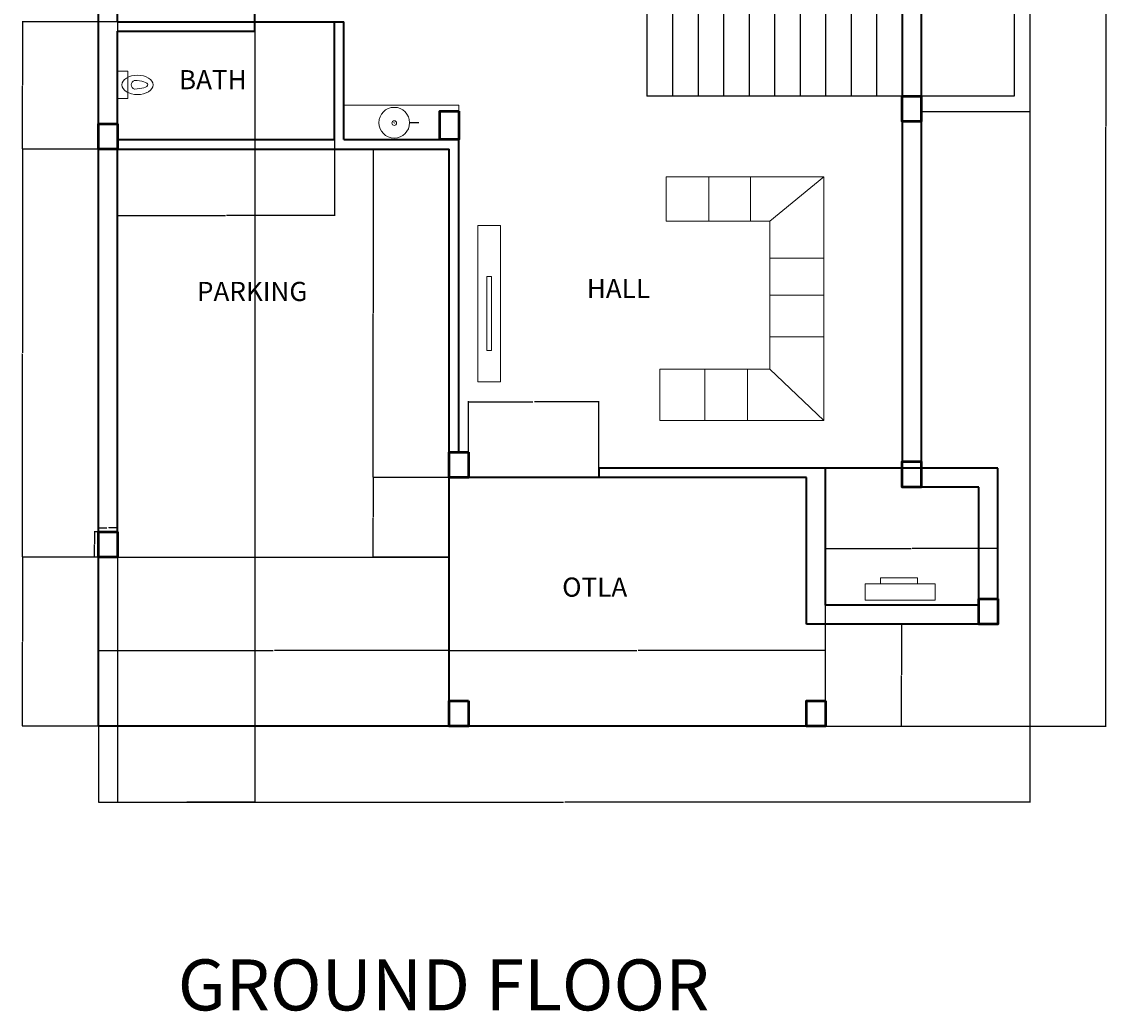
# Model space of a CAD drawing. Units: inches. Extents: x 1748 to 3019, y 1454 to 2188.
# Tile 1 of 4: x 1748 to 2258, y 1454 to 1919. Entities that reach past the tile are written whole.
import ezdxf

# ---------------------------------------------------------------- set-up
doc = ezdxf.new("R2010")
doc.units = ezdxf.units.IN
for name, color, linetype, lineweight in [('A-ANNO-DIMS', 2, 'Continuous', 18), ('A-ANNO-TEXT', 7, 'Continuous', 35), ('A-AREA-IDEN', 134, 'Continuous', 18), ('A-COLS', 120, 'Continuous', 50), ('A-FLOR', 8, 'Continuous', 25), ('A-FLOR-CASE', 9, 'Continuous', 18), ('A-WALL', 7, 'Continuous', 35), ('bathroom', 54, 'Continuous', 18), ('pooja', 117, 'Continuous', 18), ('sofa tv', 214, 'Continuous', 18), ('stairs', 64, 'Continuous', 25), ('washbasin', 106, 'Continuous', 18)]:
    doc.layers.add(name, color=color, linetype=linetype, lineweight=lineweight)
doc.styles.get("Standard").update_dxf_attribs({"font": 'arial.ttf'})
doc.dimstyles.get("Standard").update_dxf_attribs({"dimtxt": 0.18, "dimasz": 0.18, "dimexe": 0.18, "dimexo": 0.0625, "dimgap": 0.09, "dimtad": 0, "dimtih": 1, "dimtoh": 1, "dimdec": 4, "dimzin": 0, "dimdsep": 46, "dimtxsty": 'Standard', "dimcen": 0.09, "dimadec": 0, "dimazin": 0, "dimtfac": 1, "dimtdec": 4, "dimtofl": 0, "dimtmove": 0, "dimatfit": 3, "dimfxl": 1, "dimtolj": 1, "dimtzin": 0, "dimarcsym": 0})

# ---------------------------------------------------------------- blocks, each defined once
blk = doc.blocks.new('WC-CLOSE-COUPLED')
blk.add_lwpolyline([(0, 12.82), (4.89, 12.82), (4.89, 0), (0, 0)], close=True)
blk.add_arc((8.58, 6.47), 2.15, 108.3808, 251.6192)
blk.add_ellipse((9.39, 6.41), major_axis=(7.38, 0), ratio=0.615385)
blk.add_ellipse((7.39, 6.47), major_axis=(6.81, 0), ratio=0.3, start_param=4.786849, end_param=7.779521)
blk = doc.blocks.new('STAIR-FLIGHT-LANDING')
for p, q in [((0, 91.88), (129, 91.88)), ((0, 91.88), (0, 7.38)), ((12, 91.88), (12, 7.38)), ((24, 91.88), (24, 7.38)), ((36, 91.88), (36, 7.38)), ((48, 91.88), (48, 7.38)), ((60, 91.88), (60, 7.38)), ((72, 91.88), (72, 7.38)), ((84, 91.88), (84, 7.38)), ((96, 91.88), (96, 7.38)), ((108, 91.88), (108, 7.38)), ((120, 91.88), (120, 7.38)), ((0, 49.63), (120, 49.63)), ((129, 7.38), (0, 7.38))]:
    blk.add_line(p, q)
blk.add_lwpolyline([(129, 99.26), (180.11, 99.26), (180.11, 0), (129, 0)])
blk.add_lwpolyline([(129, 91.88), (172.73, 91.88), (172.73, 7.38), (129, 7.38)], close=True)
blk = doc.blocks.new('COLUMN-9X12')
blk.add_lwpolyline([(9, 12), (9, 0), (0, 0), (0, 12)], close=True)
blk = doc.blocks.new('COLUMN-RECT-EXTENDED')
blk.add_lwpolyline([(9, 13.44), (9, 0), (0, 0), (0, 13.44)], close=True)
blk = doc.blocks.new('*D8')
at = {"layer": 'A-ANNO-DIMS', "color": 0, "lineweight": -2, "transparency": 16777216}
for p, q in [((1783.72, 1679.44), (1781.8, 1679.44)), ((1781.98, 1679.26), (1781.98, 1673.62)), ((1781.98, 1667.62), (1781.98, 1673.26)), ((1783.72, 1667.44), (1781.8, 1667.44))]:
    blk.add_line(p, q, dxfattribs=at)
at = {"layer": 'A-ANNO-DIMS', "color": 0, "transparency": 16777216}
for points in [[(1781.95, 1679.26), (1782.01, 1679.26), (1781.98, 1679.44)], [(1781.95, 1667.62), (1782.01, 1667.62), (1781.98, 1667.44)]]:
    blk.add_solid(points, dxfattribs=at)
at = {"layer": 'Defpoints', "color": 0, "transparency": 16777216}
for p in [(1781.98, 1679.44), (1783.78, 1679.44), (1783.78, 1667.44)]:
    blk.add_point(p, dxfattribs=at)
at = {"layer": 'A-ANNO-DIMS', "color": 0, "transparency": 16777216, "insert": (1781.98, 1673.44), "char_height": 0.18, "attachment_point": 5}
blk.add_mtext('\\A1;COLUMN 12 TYP.', dxfattribs=at)
blk = doc.blocks.new('*D9')
at = {"layer": 'A-ANNO-DIMS', "color": 0, "lineweight": -2, "transparency": 16777216}
for p, q in [((1783.78, 1679.5), (1783.78, 1681.42)), ((1783.96, 1681.24), (1787.82, 1681.24)), ((1792.6, 1681.24), (1788.74, 1681.24)), ((1792.78, 1679.5), (1792.78, 1681.42))]:
    blk.add_line(p, q, dxfattribs=at)
at = {"layer": 'A-ANNO-DIMS', "color": 0, "transparency": 16777216}
for points in [[(1783.96, 1681.27), (1783.96, 1681.21), (1783.78, 1681.24)], [(1792.6, 1681.27), (1792.6, 1681.21), (1792.78, 1681.24)]]:
    blk.add_solid(points, dxfattribs=at)
at = {"layer": 'Defpoints', "color": 0, "transparency": 16777216}
for p in [(1783.78, 1679.44), (1792.78, 1681.24), (1792.78, 1679.44)]:
    blk.add_point(p, dxfattribs=at)
at = {"layer": 'A-ANNO-DIMS', "color": 0, "transparency": 16777216, "insert": (1788.28, 1681.24), "char_height": 0.18, "attachment_point": 5}
blk.add_mtext('\\A1;9 TYP.', dxfattribs=at)
blk = doc.blocks.new('*D22')
at = {"layer": 'A-ANNO-DIMS', "color": 0, "lineweight": -2, "transparency": 16777216}
for p, q in [((2221.89, 1877), (2221.89, 1552.06)), ((1783.78, 1587.88), (1783.78, 1552.06)), ((1783.96, 1552.24), (2002.46, 1552.24)), ((2221.71, 1552.24), (2003.22, 1552.24))]:
    blk.add_line(p, q, dxfattribs=at)
at = {"layer": 'A-ANNO-DIMS', "color": 0, "transparency": 16777216}
for points in [[(1783.96, 1552.27), (1783.96, 1552.21), (1783.78, 1552.24)], [(2221.71, 1552.27), (2221.71, 1552.21), (2221.89, 1552.24)]]:
    blk.add_solid(points, dxfattribs=at)
at = {"layer": 'Defpoints', "color": 0, "transparency": 16777216}
for p in [(2221.89, 1877.06), (1783.78, 1587.94), (2221.89, 1552.24)]:
    blk.add_point(p, dxfattribs=at)
at = {"layer": 'A-ANNO-DIMS', "color": 0, "transparency": 16777216, "insert": (2002.84, 1552.24), "char_height": 0.18, "attachment_point": 5}
blk.add_mtext('\\A1;438.1', dxfattribs=at)
blk = doc.blocks.new('*D23')
at = {"layer": 'A-ANNO-DIMS', "color": 0, "lineweight": -2, "transparency": 16777216}
for p, q in [((2170.84, 2151.94), (2257.77, 2151.94)), ((2257.59, 2151.76), (2257.59, 1870.12)), ((2257.59, 1588.12), (2257.59, 1869.76)), ((2125.84, 1587.94), (2257.77, 1587.94))]:
    blk.add_line(p, q, dxfattribs=at)
at = {"layer": 'A-ANNO-DIMS', "color": 0, "transparency": 16777216}
for points in [[(2257.56, 2151.76), (2257.62, 2151.76), (2257.59, 2151.94)], [(2257.56, 1588.12), (2257.62, 1588.12), (2257.59, 1587.94)]]:
    blk.add_solid(points, dxfattribs=at)
at = {"layer": 'Defpoints', "color": 0, "transparency": 16777216}
for p in [(2170.78, 2151.94), (2257.59, 2151.94), (2125.78, 1587.94)]:
    blk.add_point(p, dxfattribs=at)
at = {"layer": 'A-ANNO-DIMS', "color": 0, "transparency": 16777216, "insert": (2257.59, 1869.94), "char_height": 0.18, "attachment_point": 5}
blk.add_mtext('\\A1;564', dxfattribs=at)
blk = doc.blocks.new('*D27')
at = {"layer": 'A-ANNO-DIMS', "color": 0, "lineweight": -2, "transparency": 16777216}
for p, q in [((1783.72, 1859.39), (1747.9, 1859.39)), ((1748.08, 1859.21), (1748.08, 1763.6)), ((1748.08, 1667.62), (1748.08, 1763.23)), ((1783.72, 1667.44), (1747.9, 1667.44))]:
    blk.add_line(p, q, dxfattribs=at)
at = {"layer": 'A-ANNO-DIMS', "color": 0, "transparency": 16777216}
for points in [[(1748.05, 1859.21), (1748.11, 1859.21), (1748.08, 1859.39)], [(1748.05, 1667.62), (1748.11, 1667.62), (1748.08, 1667.44)]]:
    blk.add_solid(points, dxfattribs=at)
at = {"layer": 'Defpoints', "color": 0, "transparency": 16777216}
for p in [(1748.08, 1859.39), (1783.78, 1859.39), (1783.78, 1667.44)]:
    blk.add_point(p, dxfattribs=at)
at = {"layer": 'A-ANNO-DIMS', "color": 0, "transparency": 16777216, "insert": (1748.08, 1763.42), "char_height": 0.18, "attachment_point": 5}
blk.add_mtext('\\A1;191.95', dxfattribs=at)
blk = doc.blocks.new('*D28')
at = {"layer": 'A-ANNO-DIMS', "color": 0, "lineweight": -2, "transparency": 16777216}
for p, q in [((1792.72, 1919.44), (1747.9, 1919.44)), ((1748.08, 1919.26), (1748.08, 1889.6)), ((1748.08, 1859.57), (1748.08, 1889.23)), ((1792.72, 1859.39), (1747.9, 1859.39))]:
    blk.add_line(p, q, dxfattribs=at)
at = {"layer": 'A-ANNO-DIMS', "color": 0, "transparency": 16777216}
for points in [[(1748.05, 1919.26), (1748.11, 1919.26), (1748.08, 1919.44)], [(1748.05, 1859.57), (1748.11, 1859.57), (1748.08, 1859.39)]]:
    blk.add_solid(points, dxfattribs=at)
at = {"layer": 'Defpoints', "color": 0, "transparency": 16777216}
for p in [(1748.08, 1919.44), (1792.78, 1919.44), (1792.78, 1859.39)]:
    blk.add_point(p, dxfattribs=at)
at = {"layer": 'A-ANNO-DIMS', "color": 0, "transparency": 16777216, "insert": (1748.08, 1889.42), "char_height": 0.18, "attachment_point": 5}
blk.add_mtext('\\A1;60.05', dxfattribs=at)
blk = doc.blocks.new('*D31')
at = {"layer": 'A-ANNO-DIMS', "color": 0, "lineweight": -2, "transparency": 16777216}
for p, q in [((1792.78, 1970.38), (1792.78, 1552.06)), ((1857.28, 1970.38), (1857.28, 1552.06)), ((1792.96, 1552.24), (1824.71, 1552.24)), ((1857.1, 1552.24), (1825.36, 1552.24))]:
    blk.add_line(p, q, dxfattribs=at)
at = {"layer": 'A-ANNO-DIMS', "color": 0, "transparency": 16777216}
for points in [[(1792.96, 1552.27), (1792.96, 1552.21), (1792.78, 1552.24)], [(1857.1, 1552.27), (1857.1, 1552.21), (1857.28, 1552.24)]]:
    blk.add_solid(points, dxfattribs=at)
at = {"layer": 'Defpoints', "color": 0, "transparency": 16777216}
for p in [(1792.78, 1970.44), (1857.28, 1970.44), (1857.28, 1552.24)]:
    blk.add_point(p, dxfattribs=at)
at = {"layer": 'A-ANNO-DIMS', "color": 0, "transparency": 16777216, "insert": (1825.03, 1552.24), "char_height": 0.18, "attachment_point": 5}
blk.add_mtext('\\A1;64.5', dxfattribs=at)
blk = doc.blocks.new('*D32')
at = {"layer": 'A-ANNO-DIMS', "color": 0, "lineweight": -2, "transparency": 16777216}
for p, q in [((1792.78, 1863.88), (1792.78, 1828.06)), ((1894.78, 1863.88), (1894.78, 1828.06)), ((1792.96, 1828.24), (1843.5, 1828.24)), ((1894.6, 1828.24), (1844.06, 1828.24))]:
    blk.add_line(p, q, dxfattribs=at)
at = {"layer": 'A-ANNO-DIMS', "color": 0, "transparency": 16777216}
for points in [[(1792.96, 1828.27), (1792.96, 1828.21), (1792.78, 1828.24)], [(1894.6, 1828.27), (1894.6, 1828.21), (1894.78, 1828.24)]]:
    blk.add_solid(points, dxfattribs=at)
at = {"layer": 'Defpoints', "color": 0, "transparency": 16777216}
for p in [(1792.78, 1863.94), (1894.78, 1863.94), (1792.78, 1828.24)]:
    blk.add_point(p, dxfattribs=at)
at = {"layer": 'A-ANNO-DIMS', "color": 0, "transparency": 16777216, "insert": (1843.78, 1828.24), "char_height": 0.18, "attachment_point": 5}
blk.add_mtext('\\A1;102', dxfattribs=at)
blk = doc.blocks.new('*D34')
at = {"layer": 'A-ANNO-DIMS', "color": 0, "lineweight": -2, "transparency": 16777216}
for p, q in [((1948.72, 1859.44), (1912.9, 1859.44)), ((1913.08, 1859.26), (1913.08, 1782.37)), ((1913.08, 1705.12), (1913.08, 1782.01)), ((1948.72, 1704.94), (1912.9, 1704.94))]:
    blk.add_line(p, q, dxfattribs=at)
at = {"layer": 'A-ANNO-DIMS', "color": 0, "transparency": 16777216}
for points in [[(1913.05, 1859.26), (1913.11, 1859.26), (1913.08, 1859.44)], [(1913.05, 1705.12), (1913.11, 1705.12), (1913.08, 1704.94)]]:
    blk.add_solid(points, dxfattribs=at)
at = {"layer": 'Defpoints', "color": 0, "transparency": 16777216}
for p in [(1913.08, 1859.44), (1948.78, 1859.44), (1948.78, 1704.94)]:
    blk.add_point(p, dxfattribs=at)
at = {"layer": 'A-ANNO-DIMS', "color": 0, "transparency": 16777216, "insert": (1913.08, 1782.19), "char_height": 0.18, "attachment_point": 5}
blk.add_mtext('\\A1;154.5', dxfattribs=at)
blk = doc.blocks.new('*D35')
at = {"layer": 'A-ANNO-DIMS', "color": 0, "lineweight": -2, "transparency": 16777216}
for p, q in [((1783.72, 1667.44), (1747.9, 1667.44)), ((1748.08, 1667.26), (1748.08, 1627.87)), ((1748.08, 1588.12), (1748.08, 1627.51)), ((1783.72, 1587.94), (1747.9, 1587.94))]:
    blk.add_line(p, q, dxfattribs=at)
at = {"layer": 'A-ANNO-DIMS', "color": 0, "transparency": 16777216}
for points in [[(1748.05, 1667.26), (1748.11, 1667.26), (1748.08, 1667.44)], [(1748.05, 1588.12), (1748.11, 1588.12), (1748.08, 1587.94)]]:
    blk.add_solid(points, dxfattribs=at)
at = {"layer": 'Defpoints', "color": 0, "transparency": 16777216}
for p in [(1748.08, 1667.44), (1783.78, 1667.44), (1783.78, 1587.94)]:
    blk.add_point(p, dxfattribs=at)
at = {"layer": 'A-ANNO-DIMS', "color": 0, "transparency": 16777216, "insert": (1748.08, 1627.69), "char_height": 0.18, "attachment_point": 5}
blk.add_mtext('\\A1;79.5', dxfattribs=at)
blk = doc.blocks.new('*D36')
at = {"layer": 'A-ANNO-DIMS', "color": 0, "lineweight": -2, "transparency": 16777216}
for p, q in [((1783.78, 1588), (1783.78, 1623.82)), ((1783.96, 1623.64), (1866, 1623.64)), ((1948.6, 1623.64), (1866.56, 1623.64)), ((1948.78, 1588), (1948.78, 1623.82))]:
    blk.add_line(p, q, dxfattribs=at)
at = {"layer": 'A-ANNO-DIMS', "color": 0, "transparency": 16777216}
for points in [[(1783.96, 1623.67), (1783.96, 1623.61), (1783.78, 1623.64)], [(1948.6, 1623.67), (1948.6, 1623.61), (1948.78, 1623.64)]]:
    blk.add_solid(points, dxfattribs=at)
at = {"layer": 'Defpoints', "color": 0, "transparency": 16777216}
for p in [(1948.78, 1623.64), (1783.78, 1587.94), (1948.78, 1587.94)]:
    blk.add_point(p, dxfattribs=at)
at = {"layer": 'A-ANNO-DIMS', "color": 0, "transparency": 16777216, "insert": (1866.28, 1623.64), "char_height": 0.18, "attachment_point": 5}
blk.add_mtext('\\A1;165', dxfattribs=at)
blk = doc.blocks.new('*D37')
at = {"layer": 'A-ANNO-DIMS', "color": 0, "lineweight": -2, "transparency": 16777216}
for p, q in [((1948.78, 1588), (1948.78, 1623.82)), ((1948.96, 1623.64), (2037, 1623.64)), ((2125.6, 1623.64), (2037.56, 1623.64)), ((2125.78, 1588), (2125.78, 1623.82))]:
    blk.add_line(p, q, dxfattribs=at)
at = {"layer": 'A-ANNO-DIMS', "color": 0, "transparency": 16777216}
for points in [[(1948.96, 1623.67), (1948.96, 1623.61), (1948.78, 1623.64)], [(2125.6, 1623.67), (2125.6, 1623.61), (2125.78, 1623.64)]]:
    blk.add_solid(points, dxfattribs=at)
at = {"layer": 'Defpoints', "color": 0, "transparency": 16777216}
for p in [(2125.78, 1623.64), (1948.78, 1587.94), (2125.78, 1587.94)]:
    blk.add_point(p, dxfattribs=at)
at = {"layer": 'A-ANNO-DIMS', "color": 0, "transparency": 16777216, "insert": (2037.28, 1623.64), "char_height": 0.18, "attachment_point": 5}
blk.add_mtext('\\A1;177', dxfattribs=at)
blk = doc.blocks.new('*D38')
at = {"layer": 'A-ANNO-DIMS', "color": 0, "lineweight": -2, "transparency": 16777216}
for p, q in [((1948.72, 1704.94), (1912.9, 1704.94)), ((1913.08, 1704.76), (1913.08, 1686.37)), ((1913.08, 1667.62), (1913.08, 1686.01)), ((1948.72, 1667.44), (1912.9, 1667.44))]:
    blk.add_line(p, q, dxfattribs=at)
at = {"layer": 'A-ANNO-DIMS', "color": 0, "transparency": 16777216}
for points in [[(1913.05, 1704.76), (1913.11, 1704.76), (1913.08, 1704.94)], [(1913.05, 1667.62), (1913.11, 1667.62), (1913.08, 1667.44)]]:
    blk.add_solid(points, dxfattribs=at)
at = {"layer": 'Defpoints', "color": 0, "transparency": 16777216}
for p in [(1913.08, 1704.94), (1948.78, 1704.94), (1948.78, 1667.44)]:
    blk.add_point(p, dxfattribs=at)
at = {"layer": 'A-ANNO-DIMS', "color": 0, "transparency": 16777216, "insert": (1913.08, 1686.19), "char_height": 0.18, "attachment_point": 5}
blk.add_mtext('\\A1;37.5', dxfattribs=at)
blk = doc.blocks.new('*D39')
at = {"layer": 'A-ANNO-DIMS', "color": 0, "lineweight": -2, "transparency": 16777216}
for p, q in [((2125.78, 1636), (2125.78, 1671.82)), ((2125.96, 1671.64), (2166.08, 1671.64)), ((2206.6, 1671.64), (2166.48, 1671.64)), ((2206.78, 1636), (2206.78, 1671.82))]:
    blk.add_line(p, q, dxfattribs=at)
at = {"layer": 'A-ANNO-DIMS', "color": 0, "transparency": 16777216}
for points in [[(2125.96, 1671.67), (2125.96, 1671.61), (2125.78, 1671.64)], [(2206.6, 1671.67), (2206.6, 1671.61), (2206.78, 1671.64)]]:
    blk.add_solid(points, dxfattribs=at)
at = {"layer": 'Defpoints', "color": 0, "transparency": 16777216}
for p in [(2206.78, 1671.64), (2125.78, 1635.94), (2206.78, 1635.94)]:
    blk.add_point(p, dxfattribs=at)
at = {"layer": 'A-ANNO-DIMS', "color": 0, "transparency": 16777216, "insert": (2166.28, 1671.64), "char_height": 0.18, "attachment_point": 5}
blk.add_mtext('\\A1;81', dxfattribs=at)
blk = doc.blocks.new('*D40')
at = {"layer": 'A-ANNO-DIMS', "color": 0, "lineweight": -2, "transparency": 16777216}
for p, q in [((2125.84, 1635.94), (2161.66, 1635.94)), ((2161.48, 1635.76), (2161.48, 1612.12)), ((2161.48, 1588.12), (2161.48, 1611.76)), ((2125.84, 1587.94), (2161.66, 1587.94))]:
    blk.add_line(p, q, dxfattribs=at)
at = {"layer": 'A-ANNO-DIMS', "color": 0, "transparency": 16777216}
for points in [[(2161.45, 1635.76), (2161.51, 1635.76), (2161.48, 1635.94)], [(2161.45, 1588.12), (2161.51, 1588.12), (2161.48, 1587.94)]]:
    blk.add_solid(points, dxfattribs=at)
at = {"layer": 'Defpoints', "color": 0, "transparency": 16777216}
for p in [(2125.78, 1635.94), (2125.78, 1587.94), (2161.48, 1587.94)]:
    blk.add_point(p, dxfattribs=at)
at = {"layer": 'A-ANNO-DIMS', "color": 0, "transparency": 16777216, "insert": (2161.48, 1611.94), "char_height": 0.18, "attachment_point": 5}
blk.add_mtext('\\A1;48', dxfattribs=at)
blk = doc.blocks.new('*D42')
at = {"layer": 'A-ANNO-DIMS', "color": 0, "lineweight": -2, "transparency": 16777216}
for p, q in [((1957.78, 1705), (1957.78, 1740.82)), ((1957.96, 1740.64), (1988.08, 1740.64)), ((2018.98, 1740.64), (1988.87, 1740.64)), ((2019.16, 1705), (2019.16, 1740.82))]:
    blk.add_line(p, q, dxfattribs=at)
at = {"layer": 'A-ANNO-DIMS', "color": 0, "transparency": 16777216}
for points in [[(1957.96, 1740.67), (1957.96, 1740.61), (1957.78, 1740.64)], [(2018.98, 1740.67), (2018.98, 1740.61), (2019.16, 1740.64)]]:
    blk.add_solid(points, dxfattribs=at)
at = {"layer": 'Defpoints', "color": 0, "transparency": 16777216}
for p in [(2019.16, 1740.64), (1957.78, 1704.94), (2019.16, 1704.94)]:
    blk.add_point(p, dxfattribs=at)
at = {"layer": 'A-ANNO-DIMS', "color": 0, "transparency": 16777216, "insert": (1988.47, 1740.64), "char_height": 0.18, "attachment_point": 5}
blk.add_mtext('\\A1;61.38', dxfattribs=at)
blk = doc.blocks.new('*D68')
at = {"layer": 'A-ANNO-DIMS', "color": 0, "lineweight": -2, "transparency": 16777216}
for p, q in [((1922.82, 1871.9), (1923, 1871.9)), ((1922.91, 1871.81), (1922.91, 1871.99)), ((1934.48, 1871.9), (1930.33, 1871.9))]:
    blk.add_line(p, q, dxfattribs=at)
at = {"layer": 'A-ANNO-DIMS', "color": 0, "transparency": 16777216}
blk.add_solid([(1930.33, 1871.93), (1930.33, 1871.87), (1930.15, 1871.9)], dxfattribs=at)
at = {"layer": 'Defpoints', "color": 0, "transparency": 16777216}
for p in [(1915.68, 1871.9), (1930.15, 1871.9)]:
    blk.add_point(p, dxfattribs=at)
at = {"layer": 'A-ANNO-DIMS', "color": 0, "transparency": 16777216, "insert": (1935.04, 1871.9), "char_height": 0.18, "attachment_point": 5}
blk.add_mtext('\\A1;∅14.462', dxfattribs=at)

msp = doc.modelspace()

# ---------------------------------------------------------------- linework, layer by layer
at = {"layer": 'A-FLOR'}
for p, q in [((1783.7824, 1667.44), (1948.7824, 1667.44)), ((2125.7824, 1587.94), (2125.7824, 1635.94))]:
    msp.add_line(p, q, dxfattribs=at)
at = {"layer": 'A-FLOR-CASE'}
for q in [(1899.2824, 1880.2386), (1953.2824, 1877.3845)]:
    msp.add_line((1953.2824, 1880.2386), q, dxfattribs=at)
at = {"layer": 'A-WALL'}
for p, q in [((2161.7824, 2142.94), (2161.7824, 1709.44)), ((1792.7824, 1919.44), (1792.7824, 1970.44)), ((1857.2824, 1914.94), (1857.2824, 1970.44)), ((1792.7824, 1919.44), (1852.7824, 1919.44)), ((1852.7824, 1919.44), (1899.2824, 1919.44)), ((1894.7824, 1863.94), (1894.7824, 1919.44)), ((1899.2824, 1863.94), (1899.2824, 1919.44)), ((1792.7824, 1914.94), (1857.2824, 1914.94)), ((1792.7824, 1863.94), (1792.7824, 1914.94)), ((1792.7824, 1863.94), (1894.7824, 1863.94)), ((1899.2824, 1863.94), (1953.2824, 1863.94)), ((1953.2824, 1716.94), (1953.2824, 1863.94)), ((1792.7824, 1667.44), (1792.7824, 1859.44)), ((1792.7824, 1859.44), (1948.7824, 1859.44)), ((1948.7824, 1587.94), (1948.7824, 1859.44)), ((2206.7824, 1709.44), (2019.1609, 1709.44)), ((2019.1609, 1709.44), (2019.1609, 1704.94)), ((2125.7824, 1644.94), (2125.7824, 1709.44)), ((2206.7824, 1635.94), (2206.7824, 1709.44)), ((2116.7824, 1704.94), (1948.7824, 1704.94)), ((2116.7824, 1635.94), (2116.7824, 1704.94)), ((2197.7824, 1700.44), (2161.7824, 1700.44)), ((2197.7824, 1644.94), (2197.7824, 1700.44)), ((2197.7824, 1644.94), (2125.7824, 1644.94)), ((2206.7824, 1635.94), (2116.7824, 1635.94))]:
    msp.add_line(p, q, dxfattribs=at)
msp.add_lwpolyline([(2125.7824, 1587.94), (1783.7824, 1587.94), (1783.7824, 2151.94), (2170.7824, 2151.94), (2170.7824, 1709.44)], dxfattribs=at)
at = {"layer": 'pooja'}
for points in [[(2144.407, 1647.3222), (2177.3816, 1647.3222), (2177.3816, 1654.951), (2144.407, 1654.951)], [(2151.582, 1654.951), (2168.9853, 1654.951), (2168.9853, 1657.6974), (2151.582, 1657.6974)]]:
    msp.add_lwpolyline(points, close=True, dxfattribs=at)
at = {"layer": 'sofa tv'}
for p, q in [((2070.8435, 1846.3959), (2070.8435, 1825.5956)), ((2090.52, 1825.5956), (2090.52, 1846.3959)), ((2099.6015, 1825.5956), (2124.954, 1846.3959)), ((2099.6015, 1808.199), (2124.954, 1808.199)), ((2099.6015, 1790.8025), (2124.954, 1790.8025)), ((2099.6015, 1771.1368), (2124.954, 1771.1368)), ((2068.9515, 1756.0093), (2068.9515, 1731.8054)), ((2089.0064, 1756.0093), (2089.0064, 1731.8054)), ((2099.6015, 1756.0093), (2124.954, 1731.8054))]:
    msp.add_line(p, q, dxfattribs=at)
for points in [[(2099.6015, 1825.5956), (2050.7885, 1825.5956), (2050.7885, 1846.3959), (2124.954, 1846.3959), (2124.954, 1825.5956)], [(2099.6015, 1825.5956), (2099.6015, 1756.0093)], [(2124.954, 1756.0093), (2124.954, 1825.5956)], [(2099.6015, 1756.0093), (2047.7613, 1756.0093), (2047.7613, 1731.8054), (2124.954, 1731.8054), (2124.954, 1756.0093)]]:
    msp.add_lwpolyline(points, dxfattribs=at)
for points in [[(1962.2117, 1823.5687), (1972.9323, 1823.5687), (1972.9323, 1749.9947), (1962.2117, 1749.9947)], [(1966.5, 1799.5202), (1968.6441, 1799.5202), (1968.6441, 1764.7571), (1966.5, 1764.7571)]]:
    msp.add_lwpolyline(points, close=True, dxfattribs=at)
at = {"layer": 'washbasin'}
for centre, radius in [((1922.9145, 1871.9015), 7.231), ((1922.9145, 1871.7312), 1.0773)]:
    msp.add_circle(centre, radius, dxfattribs=at)

# ---------------------------------------------------------------- block references
at = {"layer": 'A-COLS'}
for name, p in [('COLUMN-9X12', (2161.782, 1872.412)), ('COLUMN-RECT-EXTENDED', (1944.282, 1863.94)), ('COLUMN-9X12', (1783.782, 1859.3932)), ('COLUMN-9X12', (1948.782, 1704.94)), ('COLUMN-9X12', (2161.782, 1700.44)), ('COLUMN-9X12', (1783.782, 1667.44)), ('COLUMN-9X12', (2197.782, 1635.94)), ('COLUMN-9X12', (1948.782, 1587.94)), ('COLUMN-9X12', (2116.782, 1587.94))]:
    msp.add_blockref(name, p, dxfattribs=at)
at = {"layer": 'bathroom'}
msp.add_blockref('WC-CLOSE-COUPLED', (1792.782, 1883.2936), dxfattribs=at)
at = {"layer": 'stairs'}
msp.add_blockref('STAIR-FLIGHT-LANDING', (2041.782, 1877.058), dxfattribs=at)

# ---------------------------------------------------------------- texts
at = {"layer": 'A-ANNO-TEXT', "insert": (1821.1127, 1478.2472), "char_height": 24, "attachment_point": 1}
msp.add_mtext_dynamic_manual_height_columns('GROUND FLOOR', width=362.834764, gutter_width=12.5, heights=[0], dxfattribs=at)
at = {"layer": 'A-AREA-IDEN', "char_height": 9, "attachment_point": 1}
for s, width, insert in [('BATH', 60.883203, (1821.672, 1896.6596)), ('PARKING', 91.929596, (1830.1435, 1797.0247)), ('HALL', 70.903152, (2013.4779, 1798.3601)), ('OTLA', 61.938386, (2001.8909, 1657.908))]:
    msp.add_mtext_dynamic_manual_height_columns(s, width=width, gutter_width=12.5, heights=[0], dxfattribs=dict(at, insert=insert))

# ---------------------------------------------------------------- dimensions: what is measured, and where the dimension line sits
at = {"layer": 'A-ANNO-DIMS'}
for base, p1, p2, angle, override, picture, middle in [((2257.5899, 2151.94), (2125.7824, 1587.94), (2170.7824, 2151.94), 90, {"dimdec": 0, "dimlfac": 1, "dimrnd": 0, "dimzin": 0, "dimdsep": 46, "dimlunit": 2}, '*D23', (2257.5899, 1869.94)), ((1748.0824, 1919.44), (1792.7824, 1859.3932), (1792.7824, 1919.44), 90, {"dimdec": 2, "dimlfac": 1, "dimrnd": 0, "dimzin": 0, "dimdsep": 46, "dimlunit": 2}, '*D28', (1748.0824, 1889.4166)), ((1792.7824, 1828.24), (1894.7824, 1863.94), (1792.7824, 1863.94), 180, {"dimdec": 0, "dimlfac": 1, "dimrnd": 0, "dimzin": 0, "dimdsep": 46, "dimlunit": 2}, '*D32', (1843.7824, 1828.24)), ((1748.0824, 1859.3932), (1783.7824, 1667.44), (1783.7824, 1859.3932), 90, {"dimdec": 2, "dimlfac": 1, "dimrnd": 0, "dimzin": 0, "dimdsep": 46, "dimlunit": 2}, '*D27', (1748.0824, 1763.4166)), ((1913.0824, 1859.44), (1948.7824, 1704.94), (1948.7824, 1859.44), 90, {"dimdec": 1, "dimlfac": 1, "dimrnd": 0, "dimzin": 0, "dimdsep": 46, "dimlunit": 2}, '*D34', (1913.0824, 1782.19)), ((1913.0824, 1704.94), (1948.7824, 1667.44), (1948.7824, 1704.94), 90, {"dimdec": 1, "dimlfac": 1, "dimrnd": 0, "dimzin": 0, "dimdsep": 46, "dimlunit": 2}, '*D38', (1913.0824, 1686.19)), ((1748.0824, 1667.44), (1783.7824, 1587.94), (1783.7824, 1667.44), 90, {"dimdec": 1, "dimlfac": 1, "dimrnd": 0, "dimzin": 0, "dimdsep": 46, "dimlunit": 2}, '*D35', (1748.0824, 1627.69)), ((2161.4824, 1587.94), (2125.7824, 1635.94), (2125.7824, 1587.94), 270, {"dimdec": 0, "dimlfac": 1, "dimrnd": 0, "dimzin": 0, "dimdsep": 46, "dimlunit": 2}, '*D40', (2161.4824, 1611.94))]:
    dim = msp.add_linear_dim(base=base, p1=p1, p2=p2, angle=angle, dimstyle='Standard', override=override, dxfattribs=at)
    dim.commit()
    dim.dimension.update_dxf_attribs({"geometry": picture, "text_midpoint": middle})
for base, p1, p2, override, picture, middle in [((1857.2824, 1552.24), (1792.7824, 1970.44), (1857.2824, 1970.44), {"dimdec": 1, "dimlfac": 1, "dimrnd": 0, "dimzin": 0, "dimdsep": 46, "dimlunit": 2}, '*D31', (1825.0324, 1552.24)), ((2221.8899, 1552.24), (1783.7824, 1587.94), (2221.8899, 1877.0584), {"dimdec": 1, "dimlfac": 1, "dimrnd": 0, "dimzin": 0, "dimdsep": 46, "dimlunit": 2}, '*D22', (2002.8361, 1552.24)), ((2019.1609, 1740.64), (1957.7824, 1704.94), (2019.1609, 1704.94), {"dimdec": 2, "dimlfac": 1, "dimrnd": 0, "dimzin": 0, "dimdsep": 46, "dimlunit": 2}, '*D42', (1988.4716, 1740.64)), ((2206.7824, 1671.64), (2125.7824, 1635.94), (2206.7824, 1635.94), {"dimdec": 0, "dimlfac": 1, "dimrnd": 0, "dimzin": 0, "dimdsep": 46, "dimlunit": 2}, '*D39', (2166.2824, 1671.64)), ((1948.7824, 1623.64), (1783.7824, 1587.94), (1948.7824, 1587.94), {"dimdec": 0, "dimlfac": 1, "dimrnd": 0, "dimzin": 0, "dimdsep": 46, "dimlunit": 2}, '*D36', (1866.2824, 1623.64)), ((2125.7824, 1623.64), (1948.7824, 1587.94), (2125.7824, 1587.94), {"dimdec": 0, "dimlfac": 1, "dimrnd": 0, "dimzin": 0, "dimdsep": 46, "dimlunit": 2}, '*D37', (2037.2824, 1623.64))]:
    dim = msp.add_linear_dim(base=base, p1=p1, p2=p2, dimstyle='Standard', override=override, dxfattribs=at)
    dim.commit()
    dim.dimension.update_dxf_attribs({"geometry": picture, "text_midpoint": middle})
dim = msp.add_diameter_dim_2p(p1=(1915.6835, 1871.902), p2=(1930.1455, 1871.901), dimstyle='Standard', override={"dimdec": 3, "dimlfac": 1, "dimrnd": 0, "dimzin": 0, "dimdsep": 46, "dimlunit": 2}, dxfattribs=at)
dim.commit()
dim.dimension.update_dxf_attribs({"geometry": '*D68', "text_midpoint": (1934.484, 1871.9007), "dimtype": 163})
dim = msp.add_linear_dim(base=(1781.9824, 1679.44), p1=(1783.7824, 1667.44), p2=(1783.7824, 1679.44), angle=90, text='COLUMN <> TYP.', dimstyle='Standard', override={"dimdec": 0, "dimlfac": 1, "dimrnd": 0, "dimzin": 0, "dimdsep": 46, "dimlunit": 2}, dxfattribs=at)
dim.commit()
dim.dimension.update_dxf_attribs({"geometry": '*D8', "text_midpoint": (1781.9824, 1673.44)})
dim = msp.add_linear_dim(base=(1792.7824, 1681.24), p1=(1783.7824, 1679.44), p2=(1792.7824, 1679.44), text='<> TYP.', dimstyle='Standard', override={"dimdec": 0, "dimlfac": 1, "dimrnd": 0, "dimzin": 0, "dimdsep": 46, "dimlunit": 2}, dxfattribs=at)
dim.commit()
dim.dimension.update_dxf_attribs({"geometry": '*D9', "text_midpoint": (1788.2824, 1681.24)})

doc.saveas('drawing.dxf')
